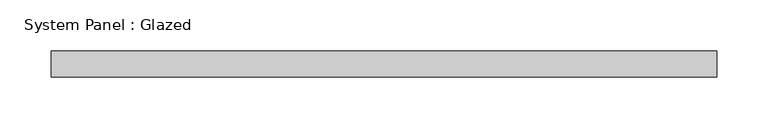
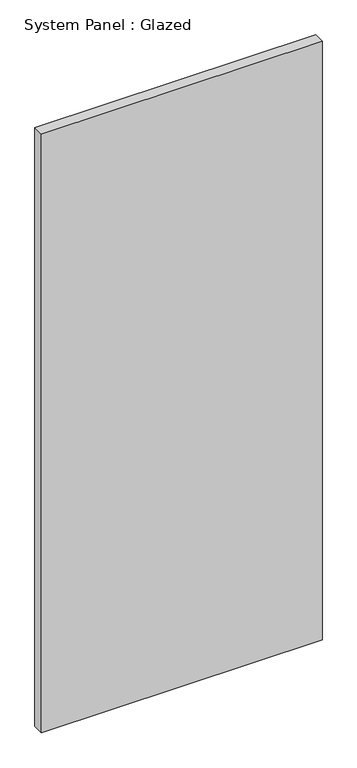
"""IFC4 building model written with IfcOpenShell, lengths in millimetres: plate geometry, System Panel : Glazed."""

from ifc_helpers import new_model, si_unit, origin, origin_with_axes, place, context, project, spatial, polyline, outline, extrude, source, transform, mapped, element, save


def system_panel_glazed_b44f8fb5(model_context):
    return source(origin(), model_context, "Body", "SweptSolid", [
        extrude(outline(polyline([(323.85, 19.05), (-323.85, 19.05), (-323.85, 44.45), (323.85, 44.45), (323.85, 19.05)])), origin_with_axes(), (0.0, 0.0, 1.0), 1460.5),
    ])


if __name__ == "__main__":
    model = new_model("IFC4")
    model_context = context("Model", 3, world=origin())
    ifc_project = project(units=[si_unit("LENGTHUNIT", "METRE", prefix="MILLI")], contexts=[model_context])
    site = spatial("IfcSite", under=ifc_project)
    building = spatial("IfcBuilding", under=site)
    placement = place(None, origin())
    system_panel_glazed_shape = system_panel_glazed_b44f8fb5(model_context)
    element("IfcPlate", 1, ObjectType="System Panel : Glazed", at=placement, inside=building, context=model_context, shape_type="MappedRepresentation", body=[
        mapped(system_panel_glazed_shape, transform((0.0, 0.0, 0.0), x_axis=(1.0, 0.0, 0.0), y_axis=(0.0, 1.0, 0.0), z_axis=(0.0, 0.0, 1.0))),
    ])
    save(model, "model.ifc")

# Revit data of these elements
# Type "System Panel : Glazed"
#   Construction Type Id = "GSP4R"
#   Analytic Construction = "1/8 in Pilkington single glazing"
#   Visual Light Transmittance = 0.9
#   Solar Heat Gain Coefficient = 0.86
#   Heat Transfer Coefficient (U) = 1.18115 BTU/(h·ft²·°F)
#   Define Thermal Properties by = 1
# Element 1 (IfcPlate, "System Panel : Glazed")
#   Materials on its faces: "Glass"
# Materials
#   "Glass": class "Glass", colour RGB 0 128 192, transparency 0.75, Description = "Soda Lime Glass", Cost = 0
